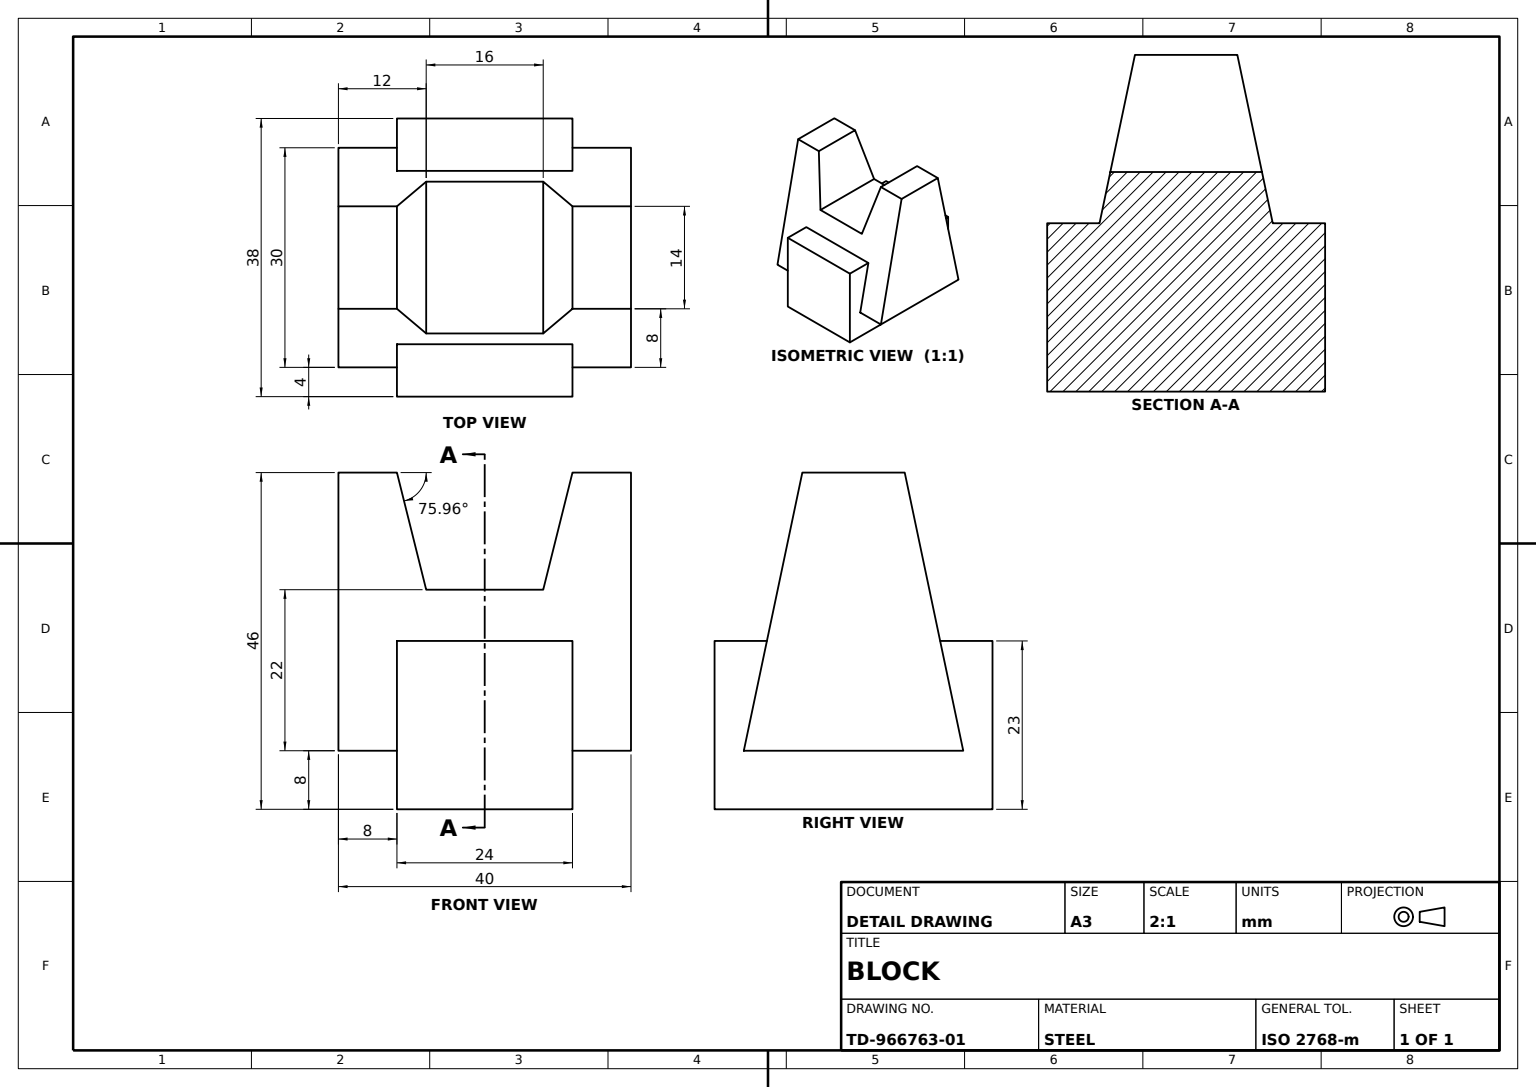
SolidWorks part; units mm, degrees
material "Plain Carbon Steel"
ref_plane "Front Plane" through (0, 0, 0) normal (0, 0, 1) x (1, 0, 0)
ref_plane "Top Plane" through (0, 0, 0) normal (0, 1, 0) x (1, 0, 0)
ref_plane "Right Plane" through (0, 0, 0) normal (1, 0, 0) x (0, 0, -1)
sketch "Base Profile Sketch" plane through (0, 0, 0) normal (0, 0, 1) x (1, 0, 0)
  line L0 (0, 48.6406) -> (0, -56.499) construction
  line L1 (56.3635, 0) -> (-64.4929, 0) construction
  line L2 (0, 0) -> (20, 0)
  line L3 (20, 0) -> (20, 38)
  line L4 (20, 38) -> (12, 38)
  line L5 (-20, 38) -> (-20, 0)
  line L6 (-20, 0) -> (0, 0)
  line L7 (20, 38) -> (20, 22)
  line L8 (8, 22) -> (-8, 22)
  line L9 (-20, 38) -> (-12, 38)
  line L10 (20, 38) -> (12, 38)
  line L11 (0, 22) -> (8, 22)
  line L12 (8, 22) -> (-8, 22)
  line L13 (-8, 22) -> (-12, 38)
  line L14 (8, 22) -> (12, 38)
  line L15 (-12, 38) -> (-20, 38)
  dimension "D2" = 12
  dimension "D1" = 8
  dimension "D3" = 22
extrude "Base Block 30mm" add sketch "Base Profile Sketch" along normal mid plane 30 contours L14 L8 L13 L9 L5 L6 L2 L3 L4
sketch "Groove Profile Sketch" plane through (0, 0, 0) normal (1, 0, 0) x (0, 0, -1)
  line L0 (-15, 0) -> (-7, 38)
  line L1 (-15, 38) -> (15, 38) construction
  line L2 (-7, 38) -> (-15, 38)
  line L3 (-15, 38) -> (-15, 0)
  line L4 (0, 44.4915) -> (0, -6.1694) construction
  line L5 (15, 38) -> (15, 0)
  line L6 (15, 0) -> (7, 38)
  line L7 (7, 38) -> (15, 38)
  dimension "D1" = 8
ref_plane "Plane2" through (20, 38, 15) normal (0, 0, -1) x (-1, 0, 0)
ref_plane "Plane3" through (20, 38, 15) normal (0, 0, -1) x (-1, 0, 0)
ref_plane "Plane4" through (20, 0, 15) normal (0, 0, -1) x (-1, 0, 0)
extrude "Groove Cut 40mm" cut sketch "Groove Profile Sketch" against normal mid plane 40 contours L0 L2 L3 | L5 L6 L7
sketch "Front Block Sketch" plane through (0, 0, 0) normal (0, 0, 1) x (1, 0, 0)
  line L0 (-12, -8) -> (-12, 15)
  line L1 (-12, 15) -> (12, 15)
  line L2 (12, 15) -> (12, -8)
  line L3 (12, -8) -> (-12, -8)
  line L4 (0, 33.8763) -> (0, -14.2655) construction
  point P6 (0, -8)
  dimension "D1" = 24
  dimension "D2" = 23
  dimension "D3" = 8
extrude "Front Block 38mm" add sketch "Front Block Sketch" along normal mid plane 38 contours L0 L1 L2 L3
